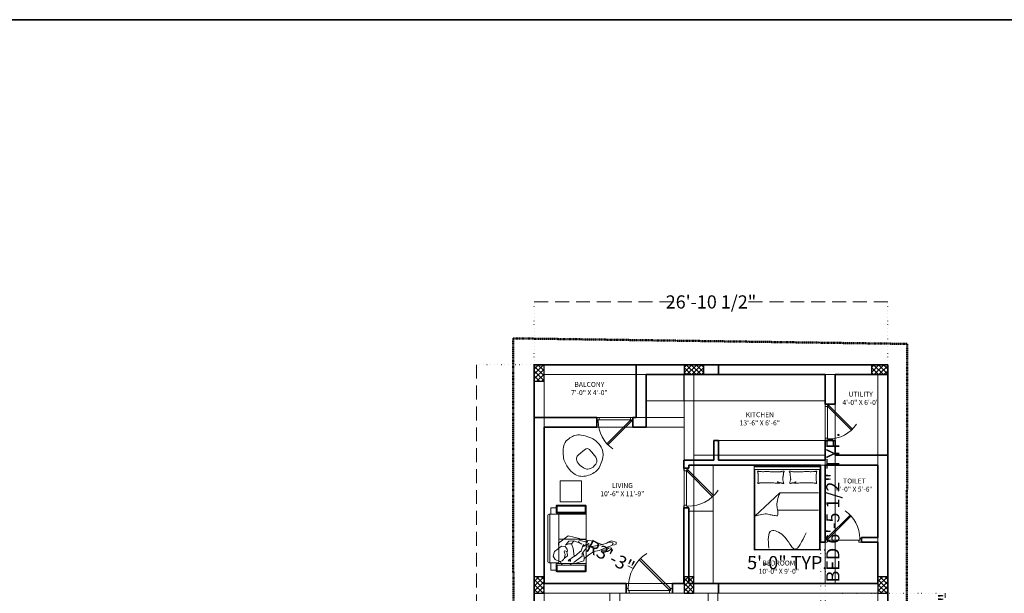
# Model space of a CAD drawing. Units: inches. Extents: x -16911 to -9621, y -48626 to -46270.
# Tile 8 of 20: x -12531 to -11633, y -47867 to -47344. Entities that reach past the tile are written whole.
import ezdxf

# ---------------------------------------------------------------- set-up
doc = ezdxf.new("R2010")
doc.units = ezdxf.units.IN
for name, pattern in [('DASHDOT', [1, 0.5, -0.25, 0, -0.25]), ('DASHED', [19.05, 12.7, -6.35]), ('DOT2', [3.175, 0, -3.175])]:
    doc.linetypes.add(name, pattern=pattern)
for name, color, linetype, lineweight in [('A-ANNO-DIMS', 2, 'Continuous', 13), ('A-AREA-IDEN', 3, 'Continuous', 18), ('A-DOOR', 4, 'Continuous', 18), ('A-FURN', 8, 'Continuous', 13), ('A-WALL', 7, 'Continuous', 35), ('C-PROP', 6, 'DASHDOT', 50), ('column', 12, 'Continuous', 30), ('DOOR', 143, 'Continuous', 9), ('EXT BEAM', 132, 'Continuous', 13), ('furniture', 35, 'Continuous', 15), ('Man', 8, 'Continuous', 5), ('S-BEAM', 132, 'Continuous', 25), ('S-COLS', 1, 'Continuous', 30)]:
    doc.layers.add(name, color=color, linetype=linetype, lineweight=lineweight)
doc.styles.add('style9', font='swisscl.ttf', dxfattribs={"height": 12})
doc.dimstyles.new('Dim9', dxfattribs={"dimtxt": 10, "dimasz": 0.199219, "dimexe": 1, "dimexo": 0.5, "dimgap": 1, "dimtad": 0, "dimdec": 1, "dimzin": 0, "dimdsep": 46, "dimlunit": 4, "dimtxsty": 'style9', "dimblk": 'ARCHTICK', "dimcen": 0.09, "dimclrd": 256, "dimclrt": 256, "dimadec": 0, "dimazin": 0, "dimtfac": 1, "dimtdec": 1, "dimtix": 1, "dimtofl": 0, "dimtmove": 1, "dimatfit": 3, "dimfxl": 9, "dimtolj": 1, "dimtzin": 0, "dimlwd": -1, "dimarcsym": 0})

# ---------------------------------------------------------------- blocks, each defined once
blk = doc.blocks.new('hjuyuiuyk')
at = {"layer": 'furniture'}
for p, q in [((-19327.49, -39738.98), (-19327.49, -39737.31)), ((-19327.49, -39737.31), (-19267.49, -39737.31, 0)), ((-19327.49, -39746.54), (-19327.49, -39737.31)), ((-19267.49, -39738.5), (-19327.49, -39738.5, 0)), ((-19327.49, -39738.5, 0), (-19327.49, -39814.72, 0)), ((-19327.49, -39738.5), (-19327.49, -39814.72)), ((-19267.49, -39738.5, 0), (-19327.49, -39738.5)), ((-19267.49, -39738.98, 0), (-19327.49, -39738.98)), ((-19268.1, -39741.33), (-19326.9, -39741.33)), ((-19326.9, -39741.33), (-19326.9, -39813.21)), ((-19268.1, -39813.21), (-19268.1, -39741.33)), ((-19267.49, -39737.31, 0), (-19267.49, -39738.98, 0)), ((-19267.49, -39746.54, 0), (-19267.49, -39737.31, 0)), ((-19267.49, -39814.72), (-19267.49, -39738.5)), ((-19267.49, -39814.72, 0), (-19267.49, -39738.5, 0)), ((-19300.88, -39753.22, 0), (-19301.49, -39750.81, 0)), ((-19300.67, -39754.09, 0), (-19300.88, -39753.22, 0)), ((-19295.19, -39754.09, 0), (-19294.97, -39753.22, 0)), ((-19294.97, -39753.22, 0), (-19294.37, -39750.81, 0)), ((-19304.07, -39762.52), (-19326.9, -39783.91)), ((-19304.07, -39762.52), (-19268.82, -39762.52)), ((-19326.9, -39813.21), (-19326.9, -39783.91)), ((-19268.82, -39778.34), (-19306.29, -39778.34)), ((-19327.49, -39814.72, 0), (-19267.49, -39814.72)), ((-19327.49, -39814.72), (-19267.49, -39814.72, 0)), ((-19269.1, -39814.21), (-19325.9, -39814.21)), ((-19325.9, -39814.21), (-19269.1, -39814.21))]:
    blk.add_line(p, q, dxfattribs=at)
for centre, radius, start, end in [((-19324.36, -39743.07, 0), 0.0997, 111.7883, 160.43603), ((-19324.39, -39743.06, 0), 0.0676, 160.43603, 281.89306), ((-19324.12, -39743.66, 0), 0.732, 94.30254, 111.7883), ((-19324.35, -39743.25, 0), 0.125, 21.9904, 101.89306), ((-19323.34, -39743.89, 0), 0.956, 158.57902, 188.13348), ((-19317.18, -39743.01, 0), 7.17, 188.13348, 192.10946), ((-19324.65, -39743.37, 0), 0.455, 338.57902, 21.9904), ((-19329.85, -39745.73, 0), 5.78, 7.6809, 12.10946), ((-19324.11, -39743.77, 0), 0.842, 59.34875, 94.30254), ((-19350.51, -39748.51, 0), 26.62, 3.36875, 7.6809), ((-19720.99, -39728.47, 0), 397.61, 356.49514, 356.94504), ((-19363.7, -39747.54, 0), 39.81, 356.94504, 358.36691), ((-19343.69, -39748.11, 0), 19.79, 358.36691, 3.36875), ((-19322.88, -39741.69, 0), 1.57, 239.34875, 264.74081), ((-19319.6, -39692.5, 0), 50.87, 266.13994, 268.60024), ((-19319.84, -39713.09, 0), 30.28, 268.09211, 271.28082), ((-19320.24, -39695.07, 0), 48.31, 271.28082, 273.40341), ((-19316.15, -39763.89, 0), 20.63, 90.1553, 93.40341), ((-19316.09, -39783.15, 0), 39.89, 86.99024, 90.1553), ((-19305.86, -39588.51, 0), 155.02, 266.99024, 268.59569), ((-19305.42, -39570.46, 0), 173.07, 268.59569, 270), ((-19305.42, -39718.38, 0), 25.15, 270, 273.68415), ((-19304.03, -39739.9, 0), 3.58, 273.68415, 287.19507), ((-19300.46, -39751.46, 0), 8.51, 98.43719, 107.19507), ((-19301.02, -39747.69, 0), 4.7, 90, 98.43719), ((-19299.57, -39750.33, 0), 1.97, 177.33512, 194.04519), ((-19282.35, -39751.13, 0), 19.21, 171.99495, 177.33512), ((-19292.22, -39749.75, 0), 9.25, 167.80162, 171.99495), ((-19326.4, -39742.36, 0), 25.72, 347.80162, 350.31563), ((-19301.12, -39743.14, 0), 0.997, 274.40021, 333.41948), ((-19315.3, -39745.68, 0), 14.34, 360, 6.23236), ((-19306.91, -39745.68, 0), 5.95, 350.31563, 360), ((-19301.02, -39745.63, 0), 2.64, 78.72762, 90), ((-19300.58, -39743.42, 0), 0.383, 333.41948, 78.72762), ((-19295.28, -39743.42, 0), 0.383, 101.27238, 206.58052), ((-19294.73, -39743.14, 0), 0.997, 206.58052, 265.59979), ((-19294.84, -39745.63, 0), 2.64, 90, 101.27238), ((-19280.55, -39745.68, 0), 14.34, 173.76764, 180), ((-19288.94, -39745.68, 0), 5.95, 180, 189.68437), ((-19294.84, -39747.69, 0), 4.7, 81.56281, 90), ((-19269.45, -39742.36, 0), 25.72, 189.68437, 192.19838), ((-19303.63, -39749.75, 0), 9.25, 8.00505, 12.19838), ((-19313.5, -39751.13, 0), 19.21, 2.66488, 8.00505), ((-19296.28, -39750.33, 0), 1.97, 345.95481, 2.66488), ((-19295.39, -39751.46, 0), 8.51, 72.80493, 81.56281), ((-19291.82, -39739.9, 0), 3.58, 252.80493, 266.31585), ((-19290.43, -39718.38, 0), 25.15, 266.31585, 270), ((-19290.43, -39570.46, 0), 173.07, 270, 271.40431), ((-19289.99, -39588.51, 0), 155.02, 271.40431, 273.00976), ((-19279.76, -39783.15, 0), 39.89, 89.8447, 93.00976), ((-19279.7, -39763.89, 0), 20.63, 86.59659, 89.8447), ((-19275.61, -39695.07, 0), 48.31, 266.59659, 268.71918), ((-19276.02, -39713.09, 0), 30.28, 268.71918, 271.90789), ((-19276.73, -39645.13, 0), 98.25, 271.00686, 272.7772), ((-19272.12, -39741.69, 0), 1.57, 275.25919, 300.65125), ((-19270.89, -39743.77, 0), 0.842, 85.69746, 120.65125), ((-19251.31, -39748.11, 0), 19.79, 176.63125, 181.63309), ((-19231.3, -39747.54, 0), 39.81, 181.63309, 183.05496), ((-19244.49, -39748.51, 0), 26.62, 172.3191, 176.63125), ((-18874.01, -39728.47, 0), 397.61, 183.05496, 183.50486), ((-19265.15, -39745.73, 0), 5.78, 167.89054, 172.3191), ((-19270.88, -39743.66, 0), 0.732, 68.2117, 85.69746), ((-19270.35, -39743.37, 0), 0.455, 158.0096, 201.42098), ((-19277.82, -39743.01, 0), 7.17, 347.89054, 351.86652), ((-19270.65, -39743.25, 0), 0.125, 78.10694, 158.0096), ((-19271.66, -39743.89, 0), 0.956, 351.86652, 21.42098), ((-19270.61, -39743.06, 0), 0.0676, 258.10694, 19.56397), ((-19270.64, -39743.07, 0), 0.0997, 19.56397, 68.2117), ((-19323.69, -39753.93, 0), 0.564, 170.00164, 196.69777), ((-19333.47, -39752.21, 0), 9.37, 350.00164, 356.49514), ((-19324.19, -39754.08, 0), 0.0385, 196.69777, 277.12039), ((-19324.51, -39751.59, 0), 2.55, 277.12039, 286.22115), ((-19324.42, -39751.9, 0), 2.23, 286.22115, 297.44392), ((-19322.81, -39754.99, 0), 1.25, 102.44799, 117.44392), ((-19322.32, -39757.22, 0), 3.54, 93.57397, 102.44799), ((-19318.44, -39837.61, 0), 84.03, 90.97549, 92.79548), ((-19315.55, -39952.16, 0), 198.61, 89.44614, 91.24735), ((-19314.9, -39885.06, 0), 131.51, 87.23256, 89.44614), ((-19310.57, -39795.48, 0), 41.81, 85.40123, 87.23256), ((-19304.32, -39717.78, 0), 36.14, 265.40123, 267.37117), ((-19297.32, -39733.09, 0), 21.54, 244.68893, 246.51559), ((-19305.66, -39747.05, 0), 6.83, 267.37117, 281.48268), ((-19297.32, -39733.09, 0), 21.54, 246.51559, 248.34226), ((-19297.32, -39733.09, 0), 21.54, 248.34226, 250.57202), ((-19297.32, -39733.09, 0), 21.54, 250.57202, 252.80178), ((-19303.46, -39757.91, 0), 4.25, 83.56595, 101.48268), ((-19303.37, -39757.16, 0), 3.49, 72.61359, 83.56595), ((-19300.33, -39747.43, 0), 6.7, 252.61359, 260.5159), ((-19300.13, -39746.25, 0), 7.9, 260.5159, 265.91706), ((-19300.69, -39754.1, 0), 0.0267, 265.91706, 14.04494), ((-19295.16, -39754.1, 0), 0.0267, 165.95506, 274.08294), ((-19295.72, -39746.25, 0), 7.9, 274.08294, 279.4841), ((-19295.52, -39747.43, 0), 6.7, 279.4841, 287.38641), ((-19292.48, -39757.16, 0), 3.49, 96.43405, 107.38641), ((-19292.39, -39757.91, 0), 4.25, 78.51732, 96.43405), ((-19298.54, -39733.09, 0), 21.54, 287.19822, 289.42798), ((-19290.19, -39747.05, 0), 6.83, 258.51732, 272.62883), ((-19298.54, -39733.09, 0), 21.54, 289.42798, 291.65774), ((-19298.54, -39733.09, 0), 21.54, 291.65774, 293.48441), ((-19298.54, -39733.09, 0), 21.54, 293.48441, 295.31107), ((-19291.53, -39717.78, 0), 36.14, 272.62883, 274.59877), ((-19285.28, -39795.48, 0), 41.81, 92.76744, 94.59877), ((-19280.95, -39885.06, 0), 131.51, 90.55386, 92.76744), ((-19280.3, -39952.16, 0), 198.61, 88.75265, 90.55386), ((-19277.1, -39805.01, 0), 51.42, 86.42603, 88.75265), ((-19274.68, -39799.75, 0), 46.07, 86.55746, 89.01709), ((-19272.19, -39754.99, 0), 1.25, 62.55608, 77.55201), ((-19270.58, -39751.9, 0), 2.23, 242.55608, 253.77885), ((-19270.49, -39751.59, 0), 2.55, 253.77885, 262.87961), ((-19261.53, -39752.21, 0), 9.37, 183.50486, 189.99836), ((-19270.81, -39754.08, 0), 0.0385, 262.87961, 343.30223), ((-19271.31, -39753.93, 0), 0.564, 343.30223, 9.99836), ((-19279.47, -39774.89), 27.53, 153.30845, 168.74227), ((-19287.94, -39773.2), 18.89, 168.74227, 187.39945), ((-19242.78, -39767.34), 64.43, 187.39945, 189.27191), ((-19306.77, -39846.83), 66.07, 105.93519, 107.73639), ((-19318.41, -39806.06), 23.67, 102.92554, 105.93519), ((-19287.64, -39956.87), 177.57, 99.72434, 101.71957), ((-19317.24, -39783.9), 2.09, 82.26962, 100.72756), ((-19317.9, -39788.76), 6.99, 76.8096, 82.26962), ((-19295.64, -39693.77), 90.57, 256.8096, 258.32586), ((-19295.11, -39691.23), 93.17, 258.32586, 260.50498), ((-19288.03, -39648.9), 136.08, 260.50498, 262.308), ((-19333.07, -39782.08), 27.05, 6.38169, 9.27191), ((-19336.71, -39780.62), 30.63, 354.11415, 359.23133), ((-19321.79, -39780.82), 15.7, 359.23133, 6.38169), ((-19325.9, -39813.21), 1, 180, 270), ((-19269.1, -39813.21), 1, 270, 0)]:
    blk.add_arc(centre, radius, start, end, dxfattribs=at)
blk.add_open_spline([(-19280.24, -39799.21), (-19283.87, -39806.94), (-19290.73, -39821.55), (-19298.08, -39801.09), (-19315.85, -39793.47), (-19314.86, -39805.92), (-19314.29, -39813.13)], degree=3, knots=[0, 0, 0, 0, 18.167809, 34.338432, 45.972904, 61.997799, 61.997799, 61.997799, 61.997799], dxfattribs=at)
blk = doc.blocks.new('Bipman02')
blk.add_lwpolyline([(0.587, -0.067), (0.618, -0.05), (0.652, -0.054), (0.67, -0.038), (0.596, 0.007), (0.544, 0.016), (0.516, 0.03), (0.496, 0.007), (0.492, -0.023), (0.452, -0.006), (0.357, 0.011), (0.292, 0.055), (0.192, 0.129), (0.187, 0.172), (0.031, 0.216), (0.005, 0.207), (-0.069, 0.246), (-0.147, 0.25), (-0.195, 0.233), (-0.225, 0.181), (-0.238, 0.185), (-0.308, 0.15), (-0.343, 0.09), (-0.325, 0.011), (-0.256, -0.037), (-0.247, -0.058), (-0.251, -0.137), (-0.086, -0.263), (0.109, -0.215), (0.109, -0.193), (0.226, -0.197), (0.231, -0.184), (0.352, -0.171), (0.409, -0.145), (0.487, -0.115), (0.509, -0.11), (0.583, -0.132), (0.609, -0.15), (0.63, -0.164), (0.661, -0.176), (0.744, -0.154), (0.748, -0.119), (0.714, -0.105), (0.674, -0.102), (0.639, -0.084)], close=True)
for points in [[(-0.256, -0.045), (-0.199, -0.084), (-0.138, -0.076), (-0.104, -0.032), (-0.099, 0.007), (-0.147, -0.002), (-0.156, 0.016), (-0.138, 0.059), (-0.151, 0.111), (-0.165, 0.15), (-0.191, 0.172), (-0.217, 0.181)], [(-0.086, 0.177), (-0.065, 0.142), (-0.052, 0.19), (-0.039, 0.129), (0.053, 0.072), (0.127, 0.003), (0.135, 0.016), (0.174, -0.106), (0.187, -0.11), (0.179, -0.076), (0.235, -0.119), (0.248, -0.106), (0.209, -0.023), (0.157, 0.042), (0.157, 0.09), (0.018, 0.194)], [(-0.156, 0.133), (-0.099, 0.085), (-0.104, 0.033), (-0.112, 0.007)], [(0.018, 0.09), (0.001, -0.041), (-0.025, -0.123), (-0.078, -0.123), (-0.13, -0.102), (-0.073, -0.167), (0.014, -0.176), (0.092, -0.145), (0.101, -0.176)], [(0.192, 0.116), (0.174, 0.037)], [(-0.025, -0.123), (0.014, -0.171)], [(0.096, -0.154), (0.153, -0.119)], [(0.27, -0.076), (0.274, -0.097), (0.27, -0.128), (0.244, -0.141), (0.222, -0.145), (0.248, -0.163), (0.248, -0.171), (0.2, -0.163), (0.114, -0.18)], [(0.231, -0.063), (0.361, -0.084), (0.509, -0.109)], [(0.492, -0.023), (0.587, -0.067)], [(0.505, -0.015), (0.552, -0.015), (0.613, -0.041)], [(0.678, -0.11), (0.691, -0.128), (0.687, -0.141), (0.657, -0.15), (0.609, -0.154)]]:
    blk.add_lwpolyline(points)
blk = doc.blocks.new('erertety')
at = {"layer": 'furniture', "ltscale": 0.2}
for p, q in [((-17662.13, -45230.66), (-17662.13, -45176.69)), ((-17693.83, -45223.2), (-17693.83, -45184.43)), ((-17685.49, -45183.68), (-17693.08, -45183.68)), ((-17684.74, -45223.2), (-17684.74, -45184.43)), ((-17684.74, -45203.31), (-17662.13, -45203.31)), ((-17685.49, -45223.95), (-17693.08, -45223.95)), ((-17691.58, -45223.95), (-17691.58, -45229.1)), ((-17684.74, -45223.99), (-17662.13, -45223.99)), ((-17684.74, -45224.55), (-17662.13, -45224.55)), ((-17684.74, -45224.55), (-17662.13, -45224.55)), ((-17691.58, -45229.1), (-17687.09, -45229.1))]:
    blk.add_line(p, q, dxfattribs=at)
for points in [[(-17662.13, -45182.17), (-17662.13, -45176.97, 0.414214), (-17662.87, -45176.22), (-17686.34, -45176.22, 0.414214), (-17687.09, -45176.97), (-17687.09, -45182.17, 0.414214), (-17686.34, -45182.91), (-17662.87, -45182.91, 0.414214)], [(-17662.13, -45225.47), (-17662.13, -45230.66, -0.414214), (-17662.87, -45231.41), (-17686.34, -45231.41, -0.414214), (-17687.09, -45230.66), (-17687.09, -45225.47, -0.414214), (-17686.34, -45224.72), (-17662.87, -45224.72, -0.414214)]]:
    blk.add_lwpolyline(points, format="xyb", close=True, dxfattribs=at)
for points in [[(-17663.01, -45181.75), (-17663.01, -45176.82), (-17686.21, -45176.82), (-17686.21, -45181.75)], [(-17692.4, -45183.68), (-17692.4, -45223.95), (-17692.4, -45223.95), (-17692.4, -45183.68)], [(-17663.01, -45225.6), (-17663.01, -45230.53), (-17686.21, -45230.53), (-17686.21, -45225.6)]]:
    blk.add_lwpolyline(points, close=True, dxfattribs=at)
blk.add_lwpolyline([(-17687.09, -45177.54), (-17691.58, -45177.54), (-17691.58, -45183.68)], dxfattribs=at)
for centre, start, end in [((-17693.08, -45184.43), 90, 180), ((-17685.49, -45184.43), 0, 90), ((-17693.08, -45223.2), 180, 270), ((-17685.49, -45223.2), 270, 0)]:
    blk.add_arc(centre, 0.748, start, end, dxfattribs=at)
at = {"layer": 'furniture', "ltscale": 0.2, "xscale": 47.90818138957024, "yscale": 47.90818138957024, "zscale": 47.90818138957024}
blk.add_blockref('Bipman02', (-17673, -45193.44, 0), dxfattribs=at)
blk = doc.blocks.new('rthrty')
at = {"layer": 'furniture'}
blk.add_open_spline([(-17650.3, -45154.53), (-17651.97, -45142.9), (-17645.3, -45136.31), (-17637.11, -45132.37), (-17620.71, -45137.17), (-17612.47, -45149.45), (-17615.73, -45159.71), (-17619.67, -45168.02), (-17632.28, -45172.65), (-17641.84, -45170.43), (-17649.5, -45159.42), (-17650.3, -45154.53)], degree=3, dxfattribs=at)
at = {"layer": 'Man'}
blk.add_open_spline([(-17632.99, -45149.02), (-17629.89, -45146.6), (-17628, -45145.12), (-17623.29, -45151.15), (-17618.06, -45156.77), (-17623.15, -45164.08), (-17628.28, -45165.32), (-17631.61, -45164.6), (-17638.01, -45159.61), (-17638.81, -45154.69), (-17636.9, -45151.81), (-17632.99, -45149.02), (-17632.99, -45149.02)], degree=3, dxfattribs=at)
blk = doc.blocks.new('A$C1C9D3E54')
at = {"layer": 'DOOR'}
blk.add_line((18676.53, 5780.72), (18710.53, 5780.72), dxfattribs=at)
blk.add_lwpolyline([(18685.01, 5806.62), (18710.47, 5781.16), (18711.53, 5782.22), (18686.07, 5807.68), (18685.01, 5806.62)], dxfattribs=at)
blk.add_lwpolyline([(18674.03, 5778.22), (18676.03, 5778.22), (18674.03, 5778.22), (18674.03, 5782.22), (18675.53, 5782.22), (18675.53, 5780.72), (18676.53, 5780.72), (18676.53, 5778.72), (18676.41, 5778.72), (18676.41, 5778.6, -0.414214), (18676.16, 5778.35), (18676.03, 5778.35), (18676.03, 5778.22)], format="xyb", dxfattribs=at)
blk.add_lwpolyline([(18713.03, 5782.22), (18711.53, 5782.22), (18711.53, 5780.72), (18710.53, 5780.72), (18710.53, 5778.72), (18710.66, 5778.72), (18710.66, 5778.6, 0.414214), (18710.91, 5778.35), (18711.03, 5778.35), (18711.03, 5778.22), (18713.03, 5778.22), (18711.03, 5778.22), (18713.03, 5778.22), (18713.03, 5782.22)], format="xyb", close=True, dxfattribs=at)
blk.add_arc((18711.53, 5782.22), 36, 124.03362, 180, dxfattribs=at)
blk = doc.blocks.new('COLUMNS')
at = {"layer": 'column'}
h = blk.add_hatch(dxfattribs=at)
h.set_pattern_fill('ANSI37', color=256, angle=-720)
h.set_pattern_definition([(45, (21703.4588, -104481.6704), (-2.24506403, 2.24506403), []), (135, (21703.4588, -104481.6704), (-2.24506403, -2.24506403), [])])
h.paths.add_polyline_path([(-12061.47, -46401.86), (-12052.47, -46401.86), (-12052.47, -46386.86), (-12061.47, -46386.86)])
h = blk.add_hatch(dxfattribs=at)
h.set_pattern_fill('ANSI37', color=256, angle=-810)
h.set_pattern_definition([(315, (-70004.5392, -80151.7886), (2.24506403, 2.24506403), []), (45, (-70004.5392, -80151.7886), (-2.24506403, 2.24506403), [])])
h.paths.add_polyline_path([(-11924.72, -46386.86), (-11924.72, -46395.86), (-11906.72, -46395.86), (-11906.72, -46386.86)])
h = blk.add_hatch(dxfattribs=at)
h.set_pattern_fill('ANSI37', color=256, angle=-810)
h.set_pattern_definition([(315, (-69833.7395, -80151.7886), (2.24506403, 2.24506403), []), (45, (-69833.7395, -80151.7886), (-2.24506403, 2.24506403), [])])
h.paths.add_polyline_path([(-11753.92, -46386.86), (-11753.92, -46395.86), (-11738.92, -46395.86), (-11738.92, -46386.86)])
h = blk.add_hatch(dxfattribs=at)
h.set_pattern_fill('ANSI37', color=256, angle=-900)
h.set_pattern_definition([(225, (-45817.4075, 11499.4594), (2.24506403, -2.24506403), []), (315, (-45817.4075, 11499.4594), (2.24506403, 2.24506403), [])])
h.paths.add_polyline_path([(-12052.47, -46580.36), (-12061.47, -46580.36), (-12061.47, -46595.36), (-12052.47, -46595.36)])
h = blk.add_hatch(dxfattribs=at)
h.set_pattern_fill('ANSI37', color=256, angle=-720)
h.set_pattern_definition([(45, (21840.2088, -104675.1704), (-2.24506403, 2.24506403), []), (135, (21840.2088, -104675.1704), (-2.24506403, -2.24506403), [])])
h.paths.add_polyline_path([(-11924.72, -46595.36), (-11915.72, -46595.36), (-11915.72, -46580.36), (-11924.72, -46580.36)])
h = blk.add_hatch(dxfattribs=at)
h.set_pattern_fill('ANSI37', color=256, angle=-900)
h.set_pattern_definition([(225, (-45503.8578, 11499.4594), (2.24506403, -2.24506403), []), (315, (-45503.8578, 11499.4594), (2.24506403, 2.24506403), [])])
h.paths.add_polyline_path([(-11738.92, -46580.36), (-11747.92, -46580.36), (-11747.92, -46595.36), (-11738.92, -46595.36)])
h = blk.add_hatch(dxfattribs=at)
h.set_pattern_fill('ANSI37', color=256, angle=-810)
h.set_pattern_definition([(315, (-70141.2892, -80432.2886), (2.24506403, 2.24506403), []), (45, (-70141.2892, -80432.2886), (-2.24506403, 2.24506403), [])])
h.paths.add_polyline_path([(-12061.47, -46667.36), (-12061.47, -46676.36), (-12046.47, -46676.36), (-12046.47, -46667.36)])
h = blk.add_hatch(dxfattribs=at)
h.set_pattern_fill('ANSI37', color=256, angle=-810)
h.set_pattern_definition([(315, (-70010.7892, -80432.2886), (2.24506403, 2.24506403), []), (45, (-70010.7892, -80432.2886), (-2.24506403, 2.24506403), [])])
h.paths.add_polyline_path([(-11930.97, -46667.36), (-11930.97, -46676.36), (-11915.97, -46676.36), (-11915.97, -46667.36)])
h = blk.add_hatch(dxfattribs=at)
h.set_pattern_fill('ANSI37', color=256, angle=-810)
h.set_pattern_definition([(315, (-69833.7395, -80432.2886), (2.24506403, 2.24506403), []), (45, (-69833.7395, -80432.2886), (-2.24506403, 2.24506403), [])])
h.paths.add_polyline_path([(-11753.92, -46667.36), (-11753.92, -46676.36), (-11738.92, -46676.36), (-11738.92, -46667.36)])
h = blk.add_hatch(dxfattribs=at)
h.set_pattern_fill('ANSI37', color=256, angle=-540)
h.set_pattern_definition([(225, (-45817.4075, 11262.5055), (2.24506403, -2.24506403), []), (315, (-45817.4075, 11262.5055), (2.24506403, 2.24506403), [])])
h.paths.add_polyline_path([(-12052.47, -46817.31), (-12061.47, -46817.31), (-12061.47, -46832.31), (-12052.47, -46832.31)])
h = blk.add_hatch(dxfattribs=at)
h.set_pattern_fill('ANSI37', color=256, angle=-720)
h.set_pattern_definition([(45, (21885.2088, -104912.1242), (-2.24506403, 2.24506403), []), (135, (21885.2088, -104912.1242), (-2.24506403, -2.24506403), [])])
h.paths.add_polyline_path([(-11879.72, -46832.31), (-11870.72, -46832.31), (-11870.72, -46817.31), (-11879.72, -46817.31)])
h = blk.add_hatch(dxfattribs=at)
h.set_pattern_fill('ANSI37', color=256, angle=-720)
h.set_pattern_definition([(45, (22017.1023, -104912.1242), (-2.24506403, 2.24506403), []), (135, (22017.1023, -104912.1242), (-2.24506403, -2.24506403), [])])
h.paths.add_polyline_path([(-11747.83, -46832.31), (-11738.83, -46832.31), (-11738.83, -46817.31), (-11747.83, -46817.31)])
h = blk.add_hatch(dxfattribs=at)
h.set_pattern_fill('ANSI37', color=256, angle=-720)
h.set_pattern_definition([(45, (21703.4588, -105024.6242), (-2.24506403, 2.24506403), []), (135, (21703.4588, -105024.6242), (-2.24506403, -2.24506403), [])])
h.paths.add_polyline_path([(-12061.47, -46944.81), (-12052.47, -46944.81), (-12052.47, -46929.81), (-12061.47, -46929.81)])
h = blk.add_hatch(dxfattribs=at)
h.set_pattern_fill('ANSI37', color=256, angle=-810)
h.set_pattern_definition([(315, (-69959.5392, -80700.7425), (2.24506403, 2.24506403), []), (45, (-69959.5392, -80700.7425), (-2.24506403, 2.24506403), [])])
h.paths.add_polyline_path([(-11879.72, -46935.81), (-11879.72, -46944.81), (-11864.72, -46944.81), (-11864.72, -46935.81)])
h = blk.add_hatch(dxfattribs=at)
h.set_pattern_fill('ANSI37', color=256, angle=-810)
h.set_pattern_definition([(315, (-69833.7395, -80700.7425), (2.24506403, 2.24506403), []), (45, (-69833.7395, -80700.7425), (-2.24506403, 2.24506403), [])])
h.paths.add_polyline_path([(-11753.92, -46935.81), (-11753.92, -46944.81), (-11738.92, -46944.81), (-11738.92, -46935.81)])
at = {"layer": 'column', "ltscale": 0.05}
for points in [[(-12052.47, -46386.86), (-12061.47, -46386.86), (-12061.47, -46401.86), (-12052.47, -46401.86)], [(-11906.72, -46395.86), (-11906.72, -46386.86), (-11924.72, -46386.86), (-11924.72, -46395.86)], [(-11738.92, -46395.86), (-11738.92, -46386.86), (-11753.92, -46386.86), (-11753.92, -46395.86)], [(-12061.47, -46595.36), (-12052.47, -46595.36), (-12052.47, -46580.36), (-12061.47, -46580.36)], [(-11915.72, -46580.36), (-11924.72, -46580.36), (-11924.72, -46595.36), (-11915.72, -46595.36)], [(-11747.92, -46595.36), (-11738.92, -46595.36), (-11738.92, -46580.36), (-11747.92, -46580.36)], [(-12046.47, -46676.36), (-12046.47, -46667.36), (-12061.47, -46667.36), (-12061.47, -46676.36)], [(-11915.97, -46676.36), (-11915.97, -46667.36), (-11930.97, -46667.36), (-11930.97, -46676.36)], [(-11738.92, -46676.36), (-11738.92, -46667.36), (-11753.92, -46667.36), (-11753.92, -46676.36)], [(-12061.47, -46832.31), (-12052.47, -46832.31), (-12052.47, -46817.31), (-12061.47, -46817.31)], [(-11870.72, -46817.31), (-11879.72, -46817.31), (-11879.72, -46832.31), (-11870.72, -46832.31)], [(-11738.83, -46817.31), (-11747.83, -46817.31), (-11747.83, -46832.31), (-11738.83, -46832.31)], [(-12052.47, -46929.81), (-12061.47, -46929.81), (-12061.47, -46944.81), (-12052.47, -46944.81)], [(-11864.72, -46944.81), (-11864.72, -46935.81), (-11879.72, -46935.81), (-11879.72, -46944.81)], [(-11738.92, -46944.81), (-11738.92, -46935.81), (-11753.92, -46935.81), (-11753.92, -46944.81)]]:
    blk.add_lwpolyline(points, close=True, dxfattribs=at)
blk = doc.blocks.new('TYPICAL BEAMS G-2')
at = {"layer": 'EXT BEAM'}
for p, q in [((-12061.47, -47658.74), (-11738.92, -47658.74)), ((-12061.47, -48216.7), (-12061.47, -47658.74)), ((-11738.92, -48216.7), (-11738.92, -47658.74)), ((-12052.47, -47667.74), (-11924.72, -47667.74)), ((-12052.47, -47939.24), (-12052.47, -47667.74)), ((-11924.72, -47667.74), (-11924.72, -47858.24)), ((-11915.72, -47667.74), (-11747.92, -47667.74)), ((-11915.72, -47667.74), (-11915.72, -47858.24)), ((-11795.92, -47667.74), (-11795.92, -47858.24)), ((-11786.92, -47667.74), (-11786.92, -47858.24)), ((-11747.92, -47858.24), (-11747.92, -47667.74)), ((-12052.47, -47706.74), (-11924.72, -47706.74)), ((-12052.47, -47715.74), (-11924.72, -47715.74)), ((-11915.72, -47741.24), (-11795.92, -47741.24)), ((-11786.92, -47741.24), (-11747.92, -47741.24)), ((-11915.72, -47750.24), (-11795.92, -47750.24)), ((-11786.92, -47750.24), (-11747.92, -47750.24)), ((-12052.47, -47858.24), (-11924.72, -47858.24)), ((-11915.72, -47858.24), (-11747.92, -47858.24)), ((-12052.47, -47867.24), (-11924.72, -47867.24)), ((-11992.47, -47867.24), (-11992.47, -47939.24)), ((-11983.47, -47867.24), (-11983.47, -47939.24)), ((-11915.72, -47867.24), (-11747.92, -47867.24)), ((-11902.92, -47867.24), (-11902.92, -47939.24)), ((-11893.92, -47867.24), (-11893.92, -47939.24)), ((-11747.92, -47939.24), (-11747.92, -47867.24)), ((-12046.47, -47939.24), (-11929.47, -47939.24)), ((-11920.47, -47939.24), (-11738.92, -47939.24)), ((-12052.47, -48089.2), (-12052.47, -47948.24)), ((-12046.47, -47948.24), (-11929.47, -47948.24)), ((-11924.97, -47948.24), (-11924.97, -48089.2)), ((-11920.47, -47948.24), (-11738.92, -47948.24)), ((-11915.97, -47948.24), (-11915.97, -48089.2)), ((-11795.92, -47948.24), (-11795.92, -48036.7)), ((-11786.92, -47948.24), (-11786.92, -48036.7)), ((-11747.92, -48089.2), (-11747.92, -47948.24)), ((-11747.92, -48036.7), (-11915.97, -48036.7)), ((-11747.92, -48045.7), (-11915.97, -48045.7)), ((-12052.47, -48089.2), (-11747.92, -48089.2)), ((-12052.47, -48216.7), (-12052.47, -48098.2)), ((-12052.47, -48098.2), (-11879.72, -48098.2)), ((-12008.97, -48098.2), (-12008.97, -48207.7)), ((-11999.97, -48098.2), (-11999.97, -48207.7)), ((-11879.72, -48098.2), (-11879.72, -48207.7)), ((-11870.72, -48098.2), (-11747.92, -48098.2)), ((-11870.72, -48098.2), (-11870.72, -48207.7)), ((-11747.92, -48207.7), (-11747.92, -48098.2)), ((-12052.47, -48207.7), (-11879.72, -48207.7)), ((-11870.72, -48207.7), (-11747.92, -48207.7)), ((-12061.47, -48216.7), (-11738.92, -48216.7))]:
    blk.add_line(p, q, dxfattribs=at)
blk = doc.blocks.new('_ArchTick')
at = {"color": 0, "linetype": 'ByBlock', "const_width": 0.15}
blk.add_lwpolyline([(-0.5, -0.5), (0.5, 0.5)], dxfattribs=at)
blk = doc.blocks.new('*D71')
at = {"layer": 'A-ANNO-DIMS', "color": 0, "linetype": 'DOT2', "lineweight": -2, "transparency": 16777216}
for p, q in [((-11800.17, -47750.24), (-11788.06, -47750.24)), ((-11800.17, -47827.65), (-11788.06, -47827.65))]:
    blk.add_line(p, q, dxfattribs=at)
at = {"layer": 'A-ANNO-DIMS', "linetype": 'DASHED', "transparency": 16777216}
for p, q in [((-11789.06, -47750.24), (-11789.06, -47750.04)), ((-11789.06, -47827.65), (-11789.06, -47827.84))]:
    blk.add_line(p, q, dxfattribs=at)
at = {"layer": 'Defpoints', "color": 0, "transparency": 16777216}
for p in [(-11800.67, -47750.24), (-11789.06, -47750.24), (-11800.67, -47827.65)]:
    blk.add_point(p, dxfattribs=at)
at = {"layer": 'A-ANNO-DIMS', "transparency": 16777216, "xscale": 0.19921875, "yscale": 0.19921875, "zscale": 0.19921875}
for p, rotation in [((-11789.06, -47750.24), 270), ((-11789.06, -47827.65), 90)]:
    blk.add_blockref('_ArchTick', p, dxfattribs=dict(at, rotation=rotation))
at = {"layer": 'A-ANNO-DIMS', "transparency": 16777216, "insert": (-11789.06, -47788.94), "char_height": 12, "attachment_point": 5, "rotation": 90, "style": 'style9'}
blk.add_mtext('\\A1;BED 6\'-5 1/2" TYP.', dxfattribs=at)
blk = doc.blocks.new('*D72')
at = {"layer": 'A-ANNO-DIMS', "color": 0, "linetype": 'DOT2', "lineweight": -2, "transparency": 16777216}
for p, q in [((-11860.67, -47828.15), (-11860.67, -47840.26)), ((-11800.67, -47828.15), (-11800.67, -47840.26))]:
    blk.add_line(p, q, dxfattribs=at)
at = {"layer": 'A-ANNO-DIMS', "linetype": 'DASHED', "transparency": 16777216}
for p, q in [((-11860.67, -47839.26), (-11859.09, -47839.26)), ((-11800.67, -47839.26), (-11802.26, -47839.26))]:
    blk.add_line(p, q, dxfattribs=at)
at = {"layer": 'Defpoints', "color": 0, "transparency": 16777216}
for p in [(-11860.67, -47827.65), (-11800.67, -47827.65), (-11800.67, -47839.26)]:
    blk.add_point(p, dxfattribs=at)
at = {"layer": 'A-ANNO-DIMS', "transparency": 16777216, "xscale": 0.19921875, "yscale": 0.19921875, "zscale": 0.19921875, "rotation": 180}
blk.add_blockref('_ArchTick', (-11860.67, -47839.26), dxfattribs=at)
at = {"layer": 'A-ANNO-DIMS', "transparency": 16777216, "xscale": 0.19921875, "yscale": 0.19921875, "zscale": 0.19921875}
blk.add_blockref('_ArchTick', (-11800.67, -47839.26), dxfattribs=at)
at = {"layer": 'A-ANNO-DIMS', "transparency": 16777216, "insert": (-11830.67, -47839.26), "char_height": 12, "attachment_point": 5, "style": 'style9'}
blk.add_mtext('\\A1;5\'-0" TYP.', dxfattribs=at)
blk = doc.blocks.new('*D119')
at = {"layer": 'A-ANNO-DIMS', "color": 0, "linetype": 'DOT2', "lineweight": -2, "transparency": 16777216}
for p, q in [((-11783.42, -47867.24), (-11685.48, -47867.24)), ((-11783.42, -47903.24), (-11685.48, -47903.24))]:
    blk.add_line(p, q, dxfattribs=at)
at = {"layer": 'A-ANNO-DIMS', "linetype": 'DASHED', "transparency": 16777216}
for p, q in [((-11686.48, -47867.24), (-11686.48, -47871.44)), ((-11686.48, -47903.24), (-11686.48, -47899.05))]:
    blk.add_line(p, q, dxfattribs=at)
at = {"layer": 'Defpoints', "color": 0, "transparency": 16777216}
for p in [(-11783.92, -47867.24), (-11783.92, -47903.24), (-11686.48, -47903.24)]:
    blk.add_point(p, dxfattribs=at)
at = {"layer": 'A-ANNO-DIMS', "transparency": 16777216, "xscale": 0.19921875, "yscale": 0.19921875, "zscale": 0.19921875}
for p, rotation in [((-11686.48, -47867.24), 90), ((-11686.48, -47903.24), 270)]:
    blk.add_blockref('_ArchTick', p, dxfattribs=dict(at, rotation=rotation))
at = {"layer": 'A-ANNO-DIMS', "transparency": 16777216, "insert": (-11686.48, -47885.24), "char_height": 12, "attachment_point": 5, "rotation": 90, "style": 'style9'}
blk.add_mtext('\\A1;3\'-0"', dxfattribs=at)
blk = doc.blocks.new('*D122')
at = {"layer": 'A-ANNO-DIMS', "color": 0, "linetype": 'DOT2', "lineweight": -2, "transparency": 16777216}
for p, q in [((-11800.42, -47821.24), (-11800.42, -48275.17)), ((-11795.92, -47821.24), (-11795.92, -48275.17))]:
    blk.add_line(p, q, dxfattribs=at)
at = {"layer": 'A-ANNO-DIMS', "linetype": 'DASHED', "transparency": 16777216}
for p, q in [((-11800.42, -48274.17), (-11800.62, -48274.17)), ((-11795.92, -48274.17), (-11795.73, -48274.17))]:
    blk.add_line(p, q, dxfattribs=at)
at = {"layer": 'Defpoints', "color": 0, "transparency": 16777216}
for p in [(-11800.42, -47820.74), (-11795.92, -47820.74), (-11795.92, -48274.17)]:
    blk.add_point(p, dxfattribs=at)
at = {"layer": 'A-ANNO-DIMS', "transparency": 16777216, "xscale": 0.19921875, "yscale": 0.19921875, "zscale": 0.19921875}
blk.add_blockref('_ArchTick', (-11800.42, -48274.17), dxfattribs=at)
at = {"layer": 'A-ANNO-DIMS', "transparency": 16777216, "xscale": 0.19921875, "yscale": 0.19921875, "zscale": 0.19921875, "rotation": 180}
blk.add_blockref('_ArchTick', (-11795.92, -48274.17), dxfattribs=at)
at = {"layer": 'A-ANNO-DIMS', "transparency": 16777216, "insert": (-11798.17, -48274.17), "char_height": 12, "attachment_point": 5, "style": 'style9'}
blk.add_mtext('\\A1;0\'-4 1/2"', dxfattribs=at)
blk = doc.blocks.new('*D131')
at = {"layer": 'A-ANNO-DIMS', "color": 0, "linetype": 'DOT2', "lineweight": -2, "transparency": 16777216}
for p, q in [((-12061.47, -47658.24), (-12061.47, -47600.45)), ((-11738.92, -47658.24), (-11738.92, -47600.45))]:
    blk.add_line(p, q, dxfattribs=at)
at = {"layer": 'A-ANNO-DIMS', "linetype": 'DASHED', "transparency": 16777216}
for p, q in [((-12061.47, -47601.45), (-11933.21, -47601.45)), ((-11738.92, -47601.45), (-11867.19, -47601.45))]:
    blk.add_line(p, q, dxfattribs=at)
at = {"layer": 'Defpoints', "color": 0, "transparency": 16777216}
for p in [(-11738.92, -47601.45), (-12061.47, -47658.74), (-11738.92, -47658.74)]:
    blk.add_point(p, dxfattribs=at)
at = {"layer": 'A-ANNO-DIMS', "transparency": 16777216, "xscale": 0.19921875, "yscale": 0.19921875, "zscale": 0.19921875, "rotation": 180}
blk.add_blockref('_ArchTick', (-12061.47, -47601.45), dxfattribs=at)
at = {"layer": 'A-ANNO-DIMS', "transparency": 16777216, "xscale": 0.19921875, "yscale": 0.19921875, "zscale": 0.19921875}
blk.add_blockref('_ArchTick', (-11738.92, -47601.45), dxfattribs=at)
at = {"layer": 'A-ANNO-DIMS', "transparency": 16777216, "insert": (-11900.2, -47601.45), "char_height": 12, "attachment_point": 5, "style": 'style9'}
blk.add_mtext('\\A1;26\'-10 1/2"', dxfattribs=at)
blk = doc.blocks.new('*D132')
at = {"layer": 'A-ANNO-DIMS', "color": 0, "linetype": 'DOT2', "lineweight": -2, "transparency": 16777216}
for p, q in [((-12061.97, -47658.74), (-12115.09, -47658.74)), ((-12061.97, -48216.7), (-12115.09, -48216.7))]:
    blk.add_line(p, q, dxfattribs=at)
at = {"layer": 'A-ANNO-DIMS', "linetype": 'DASHED', "transparency": 16777216}
for p, q in [((-12114.09, -47658.74), (-12114.09, -47920.08)), ((-12114.09, -48216.7), (-12114.09, -47955.35))]:
    blk.add_line(p, q, dxfattribs=at)
at = {"layer": 'Defpoints', "color": 0, "transparency": 16777216}
for p in [(-12061.47, -47658.74), (-12114.09, -48216.7), (-12061.47, -48216.7)]:
    blk.add_point(p, dxfattribs=at)
at = {"layer": 'A-ANNO-DIMS', "transparency": 16777216, "xscale": 0.19921875, "yscale": 0.19921875, "zscale": 0.19921875}
for p, rotation in [((-12114.09, -47658.74), 90), ((-12114.09, -48216.7), 270)]:
    blk.add_blockref('_ArchTick', p, dxfattribs=dict(at, rotation=rotation))
at = {"layer": 'A-ANNO-DIMS', "transparency": 16777216, "insert": (-12114.09, -47937.72), "char_height": 12, "attachment_point": 5, "rotation": 90, "style": 'style9'}
blk.add_mtext('\\A1;46\'-6"', dxfattribs=at)
blk = doc.blocks.new('*D135')
at = {"layer": 'A-ANNO-DIMS', "linetype": 'DASHED', "transparency": 16777216}
blk.add_line((-11976.19, -47842.17), (-11971.33, -47844.75), dxfattribs=at)
at = {"layer": 'A-ANNO-DIMS', "color": 0, "lineweight": -2, "transparency": 16777216}
for p, q in [((-11937.18, -47862.94), (-11937, -47862.94)), ((-11937.09, -47863.03), (-11937.09, -47862.85))]:
    blk.add_line(p, q, dxfattribs=at)
at = {"layer": 'Defpoints', "color": 0, "transparency": 16777216}
for p in [(-11971.33, -47844.75), (-11937.09, -47862.94)]:
    blk.add_point(p, dxfattribs=at)
at = {"layer": 'A-ANNO-DIMS', "transparency": 16777216, "xscale": 0.19921875, "yscale": 0.19921875, "zscale": 0.19921875, "rotation": 332.0173993407936}
blk.add_blockref('_ArchTick', (-11971.33, -47844.75), dxfattribs=at)
at = {"layer": 'A-ANNO-DIMS', "transparency": 16777216, "insert": (-11991.87, -47833.83), "char_height": 12, "attachment_point": 5, "rotation": 332.0174, "style": 'style9'}
blk.add_mtext('\\A1;R3\'-3"', dxfattribs=at)

msp = doc.modelspace()

# ---------------------------------------------------------------- linework, layer by layer
at = {"layer": 'A-FURN', "ltscale": 0.2}
for p, q in [((-11924.974, -47691.742), (-11924.974, -47667.742)), ((-11795.925, -47691.742), (-11959.474, -47691.742)), ((-11795.925, -47727.742), (-11893.224, -47727.742)), ((-11920.474, -47792.242), (-11898.224, -47792.242)), ((-11898.224, -47792.242), (-11898.224, -47858.242))]:
    msp.add_line(p, q, dxfattribs=at)
at = {"layer": 'A-FURN', "ltscale": 0.5}
msp.add_line((-11898.224, -47792.242), (-11898.224, -47750.242), dxfattribs=at)
at = {"layer": 'A-FURN'}
msp.add_lwpolyline([(-12018.353, -47783.864), (-12037.713, -47783.864), (-12037.713, -47764.504), (-12018.353, -47764.504)], close=True, dxfattribs=at)
at = {"layer": 'A-WALL'}
for p, q in [((-12061.474, -47706.742), (-12061.474, -47658.742)), ((-11968.474, -47658.742), (-12061.474, -47658.742)), ((-11968.474, -47706.742), (-11968.474, -47658.742)), ((-11738.925, -47658.742), (-11968.474, -47658.742)), ((-11893.506, -47658.742), (-11893.506, -47667.742)), ((-11738.925, -47658.742), (-11738.925, -47667.742)), ((-11959.474, -47715.742), (-11959.474, -47667.742)), ((-11795.925, -47667.742), (-11959.474, -47667.742)), ((-11795.925, -47667.742), (-11795.925, -47694.742)), ((-11738.925, -47667.742), (-11786.925, -47667.742)), ((-11786.925, -47667.742), (-11786.925, -47694.742)), ((-11738.925, -47667.742), (-11738.925, -47741.242)), ((-11795.925, -47694.742), (-11786.925, -47694.742)), ((-12061.474, -48168.696), (-12061.474, -47706.742)), ((-12004.474, -47706.742), (-12061.474, -47706.742)), ((-12004.474, -47706.742), (-12004.474, -47715.742)), ((-11968.474, -47706.742), (-11971.474, -47706.742)), ((-11971.474, -47706.742), (-11971.474, -47715.742)), ((-12052.474, -47858.242), (-12052.474, -47715.742)), ((-12004.474, -47715.742), (-12052.474, -47715.742)), ((-11959.474, -47715.742), (-11971.474, -47715.742)), ((-11897.724, -47745.742), (-11897.724, -47727.742)), ((-11893.224, -47727.742), (-11897.724, -47727.742)), ((-11893.224, -47745.742), (-11893.224, -47727.742)), ((-11795.925, -47727.742), (-11795.925, -47745.742)), ((-11795.925, -47727.742), (-11786.925, -47727.742)), ((-11786.925, -47727.742), (-11786.925, -47741.242)), ((-11738.925, -47741.242), (-11786.925, -47741.242)), ((-11738.925, -47741.242), (-11738.925, -47948.242)), ((-11924.974, -47753.242), (-11924.974, -47745.742)), ((-11897.724, -47745.742), (-11924.974, -47745.742)), ((-11924.974, -47753.242), (-11920.474, -47753.242)), ((-11920.474, -47753.242), (-11920.474, -47750.242)), ((-11800.425, -47750.242), (-11920.474, -47750.242)), ((-11795.925, -47745.742), (-11893.224, -47745.742)), ((-11800.425, -47750.242), (-11800.425, -47820.742)), ((-11747.925, -47750.242), (-11795.925, -47750.242)), ((-11795.925, -47750.242), (-11795.925, -47820.742)), ((-11747.925, -47750.242), (-11747.925, -47816.242)), ((-11924.974, -47858.242), (-11924.974, -47789.242)), ((-11924.974, -47789.242), (-11920.474, -47789.242)), ((-11920.474, -47858.242), (-11920.474, -47789.242)), ((-11747.925, -47816.242), (-11762.925, -47816.242)), ((-11762.925, -47816.242), (-11762.925, -47820.742)), ((-11795.925, -47820.742), (-11800.425, -47820.742)), ((-11747.925, -47820.742), (-11762.925, -47820.742)), ((-11747.925, -47820.742), (-11747.925, -47858.242)), ((-11977.474, -47858.242), (-12052.474, -47858.242)), ((-11977.474, -47867.242), (-11977.474, -47858.242)), ((-11924.974, -47858.242), (-11935.474, -47858.242)), ((-11935.474, -47867.242), (-11935.474, -47858.242)), ((-11747.925, -47858.242), (-11920.474, -47858.242)), ((-11893.506, -47858.242), (-11893.506, -47867.242)), ((-11738.925, -47858.242), (-11738.925, -47867.242))]:
    msp.add_line(p, q, dxfattribs=at)
msp.add_lwpolyline([(-13429.245, -47344.007), (-9756.987, -47344.007), (-9756.987, -48625.922), (-13429.245, -48625.922)], close=True, dxfattribs=at)
at = {"layer": 'C-PROP'}
msp.add_lwpolyline([(-12080.474, -48234.696), (-11720.293, -48240.921), (-11719.732, -48212.333), (-11720.395, -48127.492), (-11721.561, -47881.398), (-11721.175, -47639.742), (-12080.838, -47634.697), (-12080.3, -48034.841)], close=True, dxfattribs=at)

# ---------------------------------------------------------------- block references
at = {"layer": 'A-DOOR'}
for p, xscale, yscale, zscale, rotation in [((-16685.441, -63528.845), -0.8461538461538624, 0.8461538461538624, 0.8461538461538624, 270), ((-27805.577, -42817.475), -0.8461538461538624, 0.8461538461538624, 0.8461538461538624, 180), ((-17258.72, -65026.809), -0.9230769230769229, 0.9230769230769229, 0.9230769230769229, 270)]:
    msp.add_blockref('A$C1C9D3E54', p, dxfattribs=dict(at, xscale=xscale, yscale=yscale, zscale=zscale, rotation=rotation))
for p, xscale, yscale, zscale in [((4037.928, -52710.008), -0.8461538461538624, 0.8461538461538624, 0.8461538461538624), ((-32087.969, -54089.945), 1.076923076922859, 1.076923076922859, 1.076923076922859)]:
    msp.add_blockref('A$C1C9D3E54', p, dxfattribs=dict(at, xscale=xscale, yscale=yscale, zscale=zscale))
at = {"layer": 'A-FURN'}
for name, p in [('rthrty', (5615.537, -2588.962)), ('hjuyuiuyk', (7466.812, -8012.93, 0))]:
    msp.add_blockref(name, p, dxfattribs=at)
at = {"layer": 'A-FURN', "xscale": -1.1, "yscale": 1.1, "zscale": 1.1, "rotation": 180}
msp.add_blockref('erertety', (7414.285, -97541.396, 0), dxfattribs=at)
at = {"layer": 'S-BEAM'}
msp.add_blockref('TYPICAL BEAMS G-2', (0, 0), dxfattribs=at)
at = {"layer": 'S-COLS'}
msp.add_blockref('COLUMNS', (0, -1271.886), dxfattribs=at)

# ---------------------------------------------------------------- texts
at = {"layer": 'A-AREA-IDEN', "ltscale": 10, "char_height": 4.5, "width": 42.823, "attachment_point": 1, "style": 'style9'}
for s, insert in [('\\A1;\\pxqc;{\\fCentury Gothic|b0|i0|c0|p34;BALCONY\\P7\'-0" X 4\'-0"}', (-12032.568, -47674.439)), ('\\A1;\\pxqc;{\\fCentury Gothic|b0|i0|c0|p34;UTILITY\\P4\'-0" X 6\'-0"}', (-11784.997, -47683.349)), ('\\A1;\\pxqc;{\\fCentury Gothic|b0|i0|c0|p34;KITCHEN\\P13\'-6" X 6\'-6"}', (-11877.09, -47702.09)), ('\\A1;\\pxqc;{\\fCentury Gothic|b0|i0|c0|p34;TOILET\\P4\'-0" X 5\'-6"}', (-11790.748, -47762.551)), ('\\A1;\\pxqc;{\\fCentury Gothic|b0|i0|c0|p34;LIVING\\P10\'-6" X 11\'-9"}', (-12002.486, -47766.687)), ('\\A1;\\pxqc;{\\fCentury Gothic|b0|i0|c0|p34;BEDROOM\\P10\'-0" X 9\'-0"}', (-11859.726, -47837.412))]:
    msp.add_mtext(s, dxfattribs=dict(at, insert=insert))

# ---------------------------------------------------------------- dimensions: what is measured, and where the dimension line sits
at = {"layer": 'A-ANNO-DIMS'}
for base, p1, p2, picture, middle in [((-11738.925, -47601.447), (-12061.474, -47658.742), (-11738.925, -47658.742), '*D131', (-11900.199, -47601.447)), ((-11795.925, -48274.171), (-11800.425, -47820.742), (-11795.925, -47820.742), '*D122', (-11798.175, -48274.171))]:
    dim = msp.add_linear_dim(base=base, p1=p1, p2=p2, dimstyle='Dim9', override={"dimdec": 1, "dimlfac": 1, "dimrnd": 0, "dimzin": 1, "dimdsep": 46, "dimlunit": 4, "dimfrac": 2}, dxfattribs=at)
    dim.commit()
    dim.dimension.update_dxf_attribs({"geometry": picture, "text_midpoint": middle})
for base, p1, p2, picture, middle in [((-12114.088, -48216.696), (-12061.474, -47658.742), (-12061.474, -48216.696), '*D132', (-12114.088, -47937.719)), ((-11686.482, -47903.242), (-11783.925, -47867.242), (-11783.925, -47903.242), '*D119', (-11686.482, -47885.242))]:
    dim = msp.add_linear_dim(base=base, p1=p1, p2=p2, angle=90, dimstyle='Dim9', override={"dimdec": 1, "dimlfac": 1, "dimrnd": 0, "dimzin": 1, "dimdsep": 46, "dimlunit": 4, "dimfrac": 2}, dxfattribs=at)
    dim.commit()
    dim.dimension.update_dxf_attribs({"geometry": picture, "text_midpoint": middle})
dim = msp.add_linear_dim(base=(-11789.064, -47750.242), p1=(-11800.675, -47827.645), p2=(-11800.675, -47750.242), angle=90, text='BED <> TYP.', dimstyle='Dim9', override={"dimdec": 1, "dimrnd": 0, "dimzin": 1, "dimlunit": 4, "dimfrac": 2}, dxfattribs=at)
dim.commit()
dim.dimension.update_dxf_attribs({"geometry": '*D71', "text_midpoint": (-11789.064, -47788.944)})
dim = msp.add_radius_dim(center=(-11937.09, -47862.938), mpoint=(-11971.326, -47844.748), dimstyle='Dim9', override={"dimdec": 1, "dimlfac": 1, "dimrnd": 0, "dimzin": 1, "dimdsep": 46, "dimlunit": 4, "dimfrac": 2}, dxfattribs=at)
dim.commit()
dim.dimension.update_dxf_attribs({"geometry": '*D135', "text_midpoint": (-11991.868, -47833.833), "dimtype": 164})
dim = msp.add_linear_dim(base=(-11800.675, -47839.256), p1=(-11860.675, -47827.645), p2=(-11800.675, -47827.645), text='<> TYP.', dimstyle='Dim9', override={"dimdec": 1, "dimrnd": 0, "dimzin": 1, "dimlunit": 4, "dimfrac": 2}, dxfattribs=at)
dim.commit()
dim.dimension.update_dxf_attribs({"geometry": '*D72', "text_midpoint": (-11830.675, -47839.256)})

doc.saveas('drawing.dxf')
